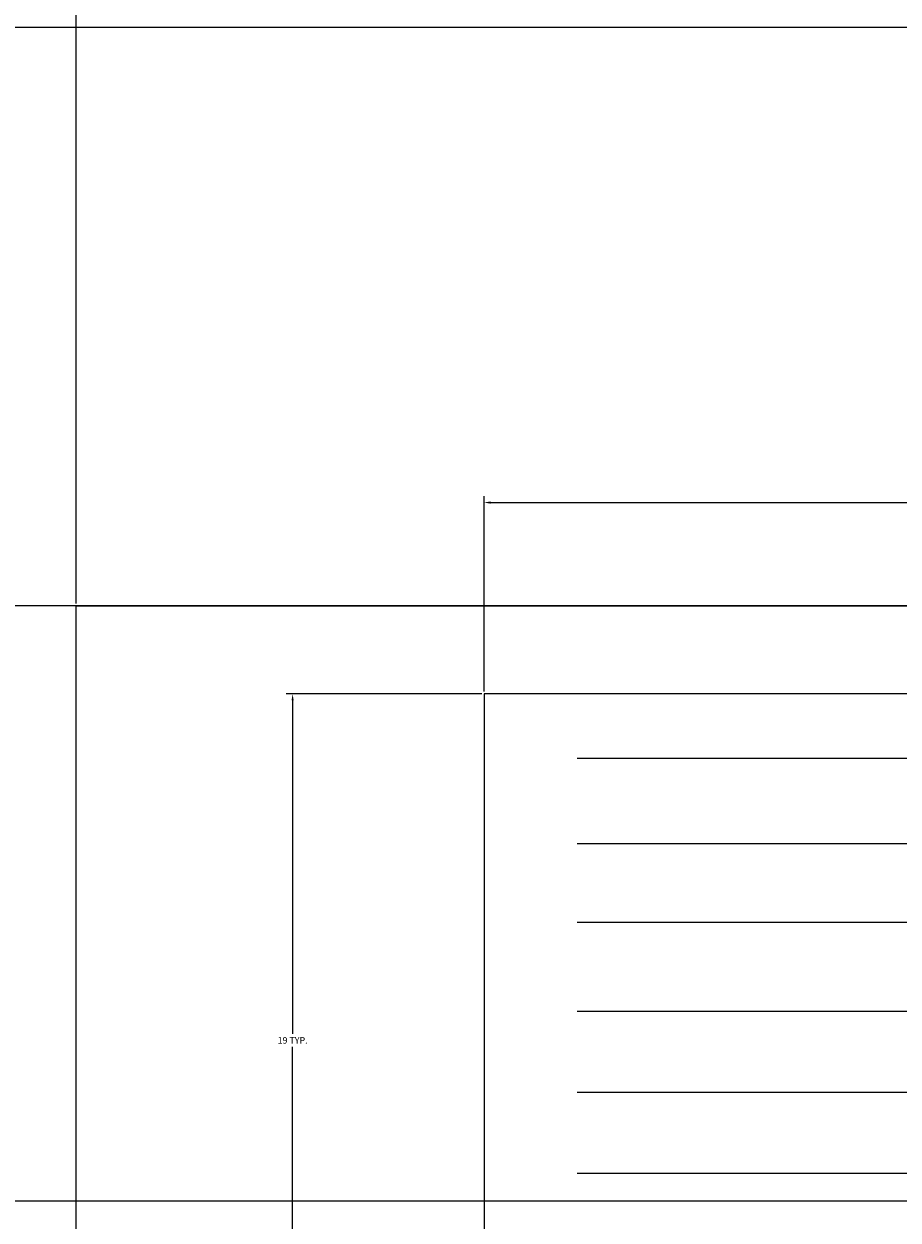
# Model space of a CAD drawing. Units: inches. Extents: x 1998 to 2588, y 1139 to 1977.
# Tile 17 of 134: x 2147 to 2171, y 1596 to 1629. Entities that reach past the tile are written whole.
import ezdxf

# ---------------------------------------------------------------- set-up
doc = ezdxf.new("R2010")
doc.units = ezdxf.units.IN
for name, color, linetype, lineweight in [('A-ANNO-DIMS', 2, 'Continuous', 18), ('A-FLOR-CASE', 32, 'Continuous', 25), ('A-FLOR-FIXT', 9, 'Continuous', 18)]:
    doc.layers.add(name, color=color, linetype=linetype, lineweight=lineweight)
doc.styles.get("Standard").update_dxf_attribs({"font": 'arial.ttf'})
doc.dimstyles.get("Standard").update_dxf_attribs({"dimtxt": 0.18, "dimasz": 0.18, "dimexe": 0.18, "dimexo": 0.0625, "dimgap": 0.09, "dimtad": 0, "dimtih": 1, "dimtoh": 1, "dimdec": 4, "dimzin": 0, "dimdsep": 46, "dimtxsty": 'Standard', "dimcen": 0.09, "dimadec": 0, "dimazin": 0, "dimtfac": 1, "dimtdec": 4, "dimtofl": 0, "dimtmove": 0, "dimatfit": 3, "dimfxl": 1, "dimtolj": 1, "dimtzin": 0, "dimarcsym": 0})

# ---------------------------------------------------------------- blocks, each defined once
blk = doc.blocks.new('SINK-WITH-DRAINBOARD')
for p, q in [((17.653, 0), (17.653, 19.174)), ((15.925, 17.391), (2.574, 17.391)), ((15.925, 15.023), (2.574, 15.023)), ((15.925, 12.848), (2.574, 12.848)), ((15.925, 10.383), (2.574, 10.383)), ((15.925, 8.143), (2.574, 8.143)), ((15.925, 5.899), (2.574, 5.899)), ((15.925, 3.752), (2.574, 3.752))]:
    blk.add_line(p, q)
blk.add_lwpolyline([(35.306, 19.174), (0, 19.174), (0, 0), (35.306, 0)], close=True)
blk.add_circle((25.956, 9.71), 1.353)
blk = doc.blocks.new('*D19')
at = {"layer": 'A-ANNO-DIMS', "color": 0, "lineweight": -2, "transparency": 16777216}
for p, q in [((2159.737, 1610.356), (2159.737, 1615.769)), ((2195.043, 1610.356), (2195.043, 1615.769)), ((2159.917, 1615.589), (2176.534, 1615.589)), ((2194.863, 1615.589), (2178.246, 1615.589))]:
    blk.add_line(p, q, dxfattribs=at)
at = {"layer": 'A-ANNO-DIMS', "color": 0, "transparency": 16777216}
for points in [[(2159.917, 1615.619), (2159.917, 1615.559), (2159.737, 1615.589)], [(2194.863, 1615.619), (2194.863, 1615.559), (2195.043, 1615.589)]]:
    blk.add_solid(points, dxfattribs=at)
at = {"layer": 'Defpoints', "color": 0, "transparency": 16777216}
for p in [(2195.043, 1615.589), (2159.737, 1610.293), (2195.043, 1610.293)]:
    blk.add_point(p, dxfattribs=at)
at = {"layer": 'A-ANNO-DIMS', "color": 0, "transparency": 16777216, "insert": (2177.39, 1615.589), "char_height": 0.18, "attachment_point": 5}
blk.add_mtext('\\A1;SINK 35 TYP.', dxfattribs=at)
blk = doc.blocks.new('*D20')
at = {"layer": 'A-ANNO-DIMS', "color": 0, "lineweight": -2, "transparency": 16777216}
for p, q in [((2159.674, 1610.293), (2154.261, 1610.293)), ((2154.441, 1610.113), (2154.441, 1600.888)), ((2154.441, 1591.299), (2154.441, 1600.524)), ((2159.674, 1591.119), (2154.261, 1591.119))]:
    blk.add_line(p, q, dxfattribs=at)
at = {"layer": 'A-ANNO-DIMS', "color": 0, "transparency": 16777216}
for points in [[(2154.411, 1610.113), (2154.471, 1610.113), (2154.441, 1610.293)], [(2154.411, 1591.299), (2154.471, 1591.299), (2154.441, 1591.119)]]:
    blk.add_solid(points, dxfattribs=at)
at = {"layer": 'Defpoints', "color": 0, "transparency": 16777216}
for p in [(2154.441, 1610.293), (2159.737, 1610.293), (2159.737, 1591.119)]:
    blk.add_point(p, dxfattribs=at)
at = {"layer": 'A-ANNO-DIMS', "color": 0, "transparency": 16777216, "insert": (2154.441, 1600.706), "char_height": 0.18, "attachment_point": 5}
blk.add_mtext('\\A1;19 TYP.', dxfattribs=at)
blk = doc.blocks.new('*D30')
at = {"layer": 'A-ANNO-DIMS', "color": 0, "lineweight": -2, "transparency": 16777216}
for p, q in [((2407.91, 1636.732), (1997.843, 1636.732)), ((1998.023, 1636.552), (1998.023, 1615.913)), ((1998.023, 1594.912), (1998.023, 1615.552)), ((2407.91, 1594.732), (1997.843, 1594.732))]:
    blk.add_line(p, q, dxfattribs=at)
at = {"layer": 'A-ANNO-DIMS', "color": 0, "transparency": 16777216}
for points in [[(1997.993, 1636.552), (1998.053, 1636.552), (1998.023, 1636.732)], [(1997.993, 1594.912), (1998.053, 1594.912), (1998.023, 1594.732)]]:
    blk.add_solid(points, dxfattribs=at)
at = {"layer": 'Defpoints', "color": 0, "transparency": 16777216}
for p in [(1998.023, 1636.732), (2407.973, 1636.732), (2407.973, 1594.732)]:
    blk.add_point(p, dxfattribs=at)
at = {"layer": 'A-ANNO-DIMS', "color": 0, "transparency": 16777216, "insert": (1998.023, 1615.732), "char_height": 0.18, "attachment_point": 5}
blk.add_mtext('\\A1;42', dxfattribs=at)
blk = doc.blocks.new('*D35')
at = {"layer": 'A-ANNO-DIMS', "color": 0, "lineweight": -2, "transparency": 16777216}
for p, q in [((2148.392, 1612.732), (1997.843, 1612.732)), ((1998.023, 1612.552), (1998.023, 1600.913)), ((1998.023, 1588.912), (1998.023, 1600.552)), ((2148.392, 1588.732), (1997.843, 1588.732))]:
    blk.add_line(p, q, dxfattribs=at)
at = {"layer": 'A-ANNO-DIMS', "color": 0, "transparency": 16777216}
for points in [[(1997.993, 1612.552), (1998.053, 1612.552), (1998.023, 1612.732)], [(1997.993, 1588.912), (1998.053, 1588.912), (1998.023, 1588.732)]]:
    blk.add_solid(points, dxfattribs=at)
at = {"layer": 'Defpoints', "color": 0, "transparency": 16777216}
for p in [(1998.023, 1612.732), (2148.455, 1612.732), (2148.455, 1588.732)]:
    blk.add_point(p, dxfattribs=at)
at = {"layer": 'A-ANNO-DIMS', "color": 0, "transparency": 16777216, "insert": (1998.023, 1600.732), "char_height": 0.18, "attachment_point": 5}
blk.add_mtext('\\A1;24', dxfattribs=at)
blk = doc.blocks.new('*D37')
at = {"layer": 'A-ANNO-DIMS', "color": 0, "lineweight": -2, "transparency": 16777216}
for p, q in [((2148.455, 1612.795), (2148.455, 1977.362)), ((2148.635, 1977.182), (2172.73, 1977.182)), ((2197.27, 1977.182), (2173.175, 1977.182)), ((2197.45, 1612.795), (2197.45, 1977.362))]:
    blk.add_line(p, q, dxfattribs=at)
at = {"layer": 'A-ANNO-DIMS', "color": 0, "transparency": 16777216}
for points in [[(2148.635, 1977.212), (2148.635, 1977.152), (2148.455, 1977.182)], [(2197.27, 1977.212), (2197.27, 1977.152), (2197.45, 1977.182)]]:
    blk.add_solid(points, dxfattribs=at)
at = {"layer": 'Defpoints', "color": 0, "transparency": 16777216}
for p in [(2197.45, 1977.182), (2148.455, 1612.732), (2197.45, 1612.732)]:
    blk.add_point(p, dxfattribs=at)
at = {"layer": 'A-ANNO-DIMS', "color": 0, "transparency": 16777216, "insert": (2172.952, 1977.182), "char_height": 0.18, "attachment_point": 5}
blk.add_mtext('\\A1;49', dxfattribs=at)
blk = doc.blocks.new('*D38')
at = {"layer": 'A-ANNO-DIMS', "color": 0, "lineweight": -2, "transparency": 16777216}
for p, q in [((2197.387, 1663.247), (1997.843, 1663.247)), ((1998.023, 1663.067), (1998.023, 1638.171)), ((1998.023, 1612.912), (1998.023, 1637.808)), ((2197.387, 1612.732), (1997.843, 1612.732))]:
    blk.add_line(p, q, dxfattribs=at)
at = {"layer": 'A-ANNO-DIMS', "color": 0, "transparency": 16777216}
for points in [[(1997.993, 1663.067), (1998.053, 1663.067), (1998.023, 1663.247)], [(1997.993, 1612.912), (1998.053, 1612.912), (1998.023, 1612.732)]]:
    blk.add_solid(points, dxfattribs=at)
at = {"layer": 'Defpoints', "color": 0, "transparency": 16777216}
for p in [(1998.023, 1663.247), (2197.45, 1663.247), (2197.45, 1612.732)]:
    blk.add_point(p, dxfattribs=at)
at = {"layer": 'A-ANNO-DIMS', "color": 0, "transparency": 16777216, "insert": (1998.023, 1637.99), "char_height": 0.18, "attachment_point": 5}
blk.add_mtext('\\A1;50.51', dxfattribs=at)
blk = doc.blocks.new('*D39')
at = {"layer": 'A-ANNO-DIMS', "color": 0, "lineweight": -2, "transparency": 16777216}
for p, q in [((2115.035, 1628.742), (2588.309, 1628.742)), ((2588.129, 1628.562), (2588.129, 1612.685)), ((2588.129, 1596.444), (2588.129, 1612.321)), ((2115.035, 1596.264), (2588.309, 1596.264))]:
    blk.add_line(p, q, dxfattribs=at)
at = {"layer": 'A-ANNO-DIMS', "color": 0, "transparency": 16777216}
for points in [[(2588.099, 1628.562), (2588.159, 1628.562), (2588.129, 1628.742)], [(2588.099, 1596.444), (2588.159, 1596.444), (2588.129, 1596.264)]]:
    blk.add_solid(points, dxfattribs=at)
at = {"layer": 'Defpoints', "color": 0, "transparency": 16777216}
for p in [(2114.973, 1628.742), (2588.129, 1628.742), (2114.973, 1596.264)]:
    blk.add_point(p, dxfattribs=at)
at = {"layer": 'A-ANNO-DIMS', "color": 0, "transparency": 16777216, "insert": (2588.129, 1612.503), "char_height": 0.18, "attachment_point": 5}
blk.add_mtext('\\A1;32.48', dxfattribs=at)

msp = doc.modelspace()

# ---------------------------------------------------------------- linework, layer by layer
at = {"layer": 'A-FLOR-CASE'}
for p, q in [((2148.4548, 1588.7324), (2148.4548, 1612.7324)), ((2148.4548, 1612.7324), (2197.4499, 1612.7324))]:
    msp.add_line(p, q, dxfattribs=at)

# ---------------------------------------------------------------- block references
at = {"layer": 'A-FLOR-FIXT'}
msp.add_blockref('SINK-WITH-DRAINBOARD', (2159.737, 1591.119), dxfattribs=at)

# ---------------------------------------------------------------- dimensions: what is measured, and where the dimension line sits
at = {"layer": 'A-ANNO-DIMS'}
dim = msp.add_linear_dim(base=(2197.4499, 1977.1824), p1=(2148.4548, 1612.7324), p2=(2197.4499, 1612.7324), dimstyle='Standard', override={"dimdec": 0, "dimlfac": 1, "dimrnd": 0, "dimzin": 0, "dimdsep": 46, "dimlunit": 2}, dxfattribs=at)
dim.commit()
dim.dimension.update_dxf_attribs({"geometry": '*D37', "text_midpoint": (2172.9524, 1977.1824)})
for base, p1, p2, override, picture, middle in [((1998.0229, 1663.2466), (2197.4499, 1612.7324), (2197.4499, 1663.2466), {"dimdec": 2, "dimlfac": 1, "dimrnd": 0, "dimzin": 0, "dimdsep": 46, "dimlunit": 2}, '*D38', (1998.0229, 1637.9895)), ((1998.0229, 1636.7324), (2407.9729, 1594.7324), (2407.9729, 1636.7324), {"dimdec": 0, "dimlfac": 1, "dimrnd": 0, "dimzin": 0, "dimdsep": 46, "dimlunit": 2}, '*D30', (1998.0229, 1615.7324)), ((2588.1286, 1628.7416), (2114.9729, 1596.2642), (2114.9729, 1628.7416), {"dimdec": 2, "dimlfac": 1, "dimrnd": 0, "dimzin": 0, "dimdsep": 46, "dimlunit": 2}, '*D39', (2588.1286, 1612.5029)), ((1998.0229, 1612.7324), (2148.4548, 1588.7324), (2148.4548, 1612.7324), {"dimdec": 0, "dimlfac": 1, "dimrnd": 0, "dimzin": 0, "dimdsep": 46, "dimlunit": 2}, '*D35', (1998.0229, 1600.7324))]:
    dim = msp.add_linear_dim(base=base, p1=p1, p2=p2, angle=90, dimstyle='Standard', override=override, dxfattribs=at)
    dim.commit()
    dim.dimension.update_dxf_attribs({"geometry": picture, "text_midpoint": middle})
dim = msp.add_linear_dim(base=(2195.0425, 1615.5894), p1=(2159.7366, 1610.2935), p2=(2195.0425, 1610.2935), text='SINK <> TYP.', dimstyle='Standard', override={"dimdec": 0, "dimlfac": 1, "dimrnd": 0, "dimzin": 0, "dimdsep": 46, "dimlunit": 2}, dxfattribs=at)
dim.commit()
dim.dimension.update_dxf_attribs({"geometry": '*D19', "text_midpoint": (2177.3896, 1615.5894)})
dim = msp.add_linear_dim(base=(2154.4407, 1610.2935), p1=(2159.7366, 1591.1193), p2=(2159.7366, 1610.2935), angle=90, text='<> TYP.', dimstyle='Standard', override={"dimdec": 0, "dimlfac": 1, "dimrnd": 0, "dimzin": 0, "dimdsep": 46, "dimlunit": 2}, dxfattribs=at)
dim.commit()
dim.dimension.update_dxf_attribs({"geometry": '*D20', "text_midpoint": (2154.4407, 1600.7064)})

doc.saveas('drawing.dxf')
